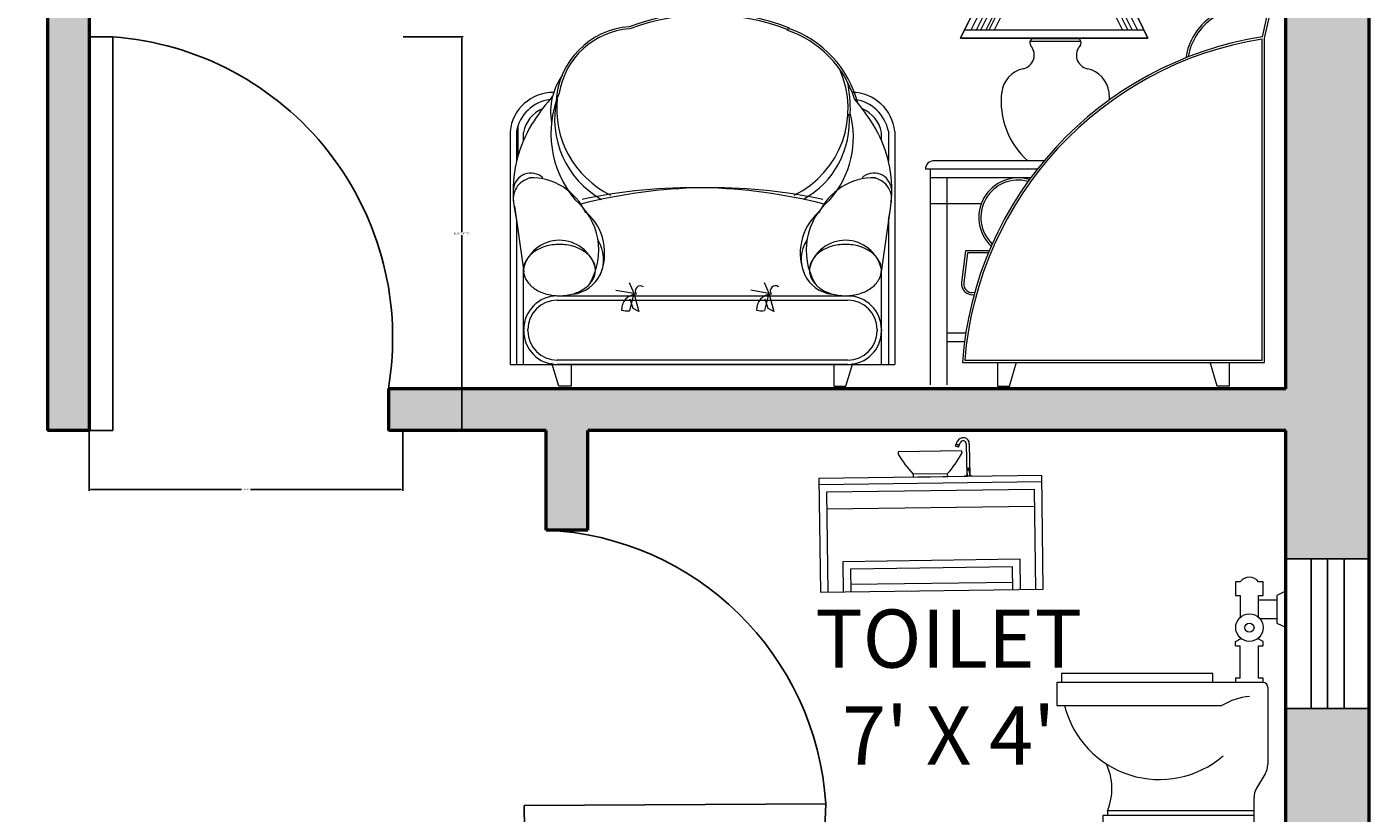
# Model space of a CAD drawing. Units: inches. Extents: x 1771 to 3025, y 319 to 889.
# Tile 30 of 35: x 2863 to 3025, y 619 to 714. Entities that reach past the tile are written whole.
import ezdxf

# ---------------------------------------------------------------- set-up
doc = ezdxf.new("R2010")
doc.units = ezdxf.units.IN
doc.header["$MEASUREMENT"] = 0
doc.set_wipeout_variables(frame=1)
for name, color, linetype, lineweight in [('A-ANNO-DIMS', 2, 'Continuous', 18), ('A-AREA-IDEN', 241, 'Continuous', 25), ('A-DOOR', 4, 'Continuous', 25), ('A-FLOR-FIXT', 8, 'Continuous', 18), ('A-FURN', 8, 'Continuous', 18), ('A-GLAZ', 40, 'Continuous', 25), ('A-WALL', 7, 'Continuous', 50), ('A-WALL-PATT', 254, 'Continuous', 13)]:
    doc.layers.add(name, color=color, linetype=linetype, lineweight=lineweight)
doc.styles.get("Standard").update_dxf_attribs({"font": 'arial.ttf'})
doc.dimstyles.get("Standard").update_dxf_attribs({"dimtxt": 0.18, "dimasz": 0.18, "dimexe": 0.18, "dimexo": 0.0625, "dimgap": 0.09, "dimtad": 0, "dimtih": 1, "dimtoh": 1, "dimdec": 4, "dimzin": 0, "dimdsep": 46, "dimtxsty": 'Standard', "dimcen": 0.09, "dimadec": 0, "dimazin": 0, "dimtfac": 1, "dimtdec": 4, "dimtofl": 0, "dimtmove": 0, "dimatfit": 3, "dimfxl": 1, "dimtolj": 1, "dimtzin": 0, "dimarcsym": 0})

# ---------------------------------------------------------------- blocks, each defined once
blk = doc.blocks.new('A$C425441F1')
for points in [[(1639.3, 0), (1667.3, 0), (1667.3, 55.3), (1748.6, 55.3), (1748.6, 807.4), (1761.1, 860.7), (1735.7, 880.7), (1703.4, 883.3), (1675.8, 879.6), (1656.2, 873.5), (1635.2, 863.3), (1619.6, 852.6), (1605.1, 839.5), (1596.7, 829.9), (1583.2, 810), (1573.2, 788.1), (1567.6, 767.7), (1566.5, 761.6), (1541.6, 750.9), (1510.7, 736.6), (1488.3, 725.3), (1464.5, 712.2), (1433.4, 693.6), (1409.1, 677.8), (1389.7, 664.2), (1388.2, 683.8), (1383.3, 700), (1376.2, 712), (1365.5, 723.2), (1352, 731.8), (1342.1, 735.4), (1331.7, 738.6), (1325, 742.7), (1317.7, 750.9), (1314.2, 758.8), (1312.9, 767.9), (1315.6, 780.8), (1321.1, 788.9), (1323.4, 793.7), (1323.6, 797.2), (1323.1, 800), (1320.5, 804.5), (1317.8, 806.7), (1317.8, 807.1), (1478.8, 807.1), (1345.8, 1080.7), (1177.3, 1080.7), (1044.3, 807.1), (1211.1, 807.1), (1211.1, 806.7), (1207.8, 803.9), (1205.8, 800.4), (1205.1, 796.3), (1207.6, 788.9), (1211.4, 783.4), (1213.5, 778.7), (1215.3, 769.8), (1215.1, 763.9), (1214.1, 759), (1208.8, 748.5), (1201.9, 741.7), (1195.3, 738), (1185.9, 735.4), (1176, 731.7), (1166.8, 726.4), (1159.9, 720.8), (1156.8, 717.7), (1149.3, 708.1), (1145.7, 701.6), (1143.6, 696.9), (1138.7, 669.7), (1138.7, 651.6), (1140.7, 631.8), (1142.6, 621.6), (1148.5, 600.5), (1162.8, 569), (1176.9, 547.8), (1188.6, 534.2), (1200, 523), (983, 523), (977.7, 522.3), (971.8, 519.6), (965.5, 512.8), (963.3, 506.8), (963, 503), (974.8, 503), (974.8, 3), (1013, 3), (1013, 103), (1053.6, 103), (1052.7, 96.1), (1051.6, 86.5), (1049.3, 63.6), (1048.6, 55.3), (1130.1, 55.3), (1130.1, 0), (1157.9, 0), (1174.1, 55.3), (1623.1, 55.6)], [(778.6, 0), (750.6, 0), (750.6, 50.4), (141.4, 50.4), (141.4, 0), (113.4, 0), (98.1, 50.4), (0, 50.4), (0, 590.4), (3.6, 609.1), (14.7, 633.7), (36.6, 658.7), (60.6, 673.3), (86.6, 680.5), (100.5, 681.5), (107.8, 698), (118.3, 717), (136.4, 751.3), (159.1, 779.5), (188.4, 803.6), (213.2, 817.4), (239.4, 827.1), (258.7, 831.4), (276, 833.4), (301.1, 842.1), (332.2, 850.9), (368.4, 858.6), (403.3, 863.5), (432.7, 865.8), (472.6, 866.2), (499.3, 864.8), (525, 862.1), (551.9, 857.9), (572.9, 853.6), (591.1, 849.1), (612.6, 842.8), (648, 830.4), (661.5, 823.7), (679.5, 815.2), (707.5, 798.2), (726.7, 783.3), (755.4, 754.4), (773.7, 729.8), (788.1, 704.9), (796.6, 686.1), (798.5, 681.2), (818, 677.9), (833.5, 672.3), (851.7, 661.6), (864.4, 650.3), (878.3, 632.1), (887.5, 611.7), (891.4, 595.2), (892, 590.4), (892, 50.4), (793.9, 50.4)]]:
    blk.add_wipeout(points)
for p, q in [((1044.3, 807.1), (1177.3, 1080.7)), ((1177.3, 1080.7), (1044.3, 807.1)), ((1188.8, 1068), (1069.3, 827.4)), ((1201.1, 1068), (1081.6, 827.4)), ((1211.2, 1068), (1091.7, 827.4)), ((1223.5, 1068), (1104, 827.4)), ((1230.5, 1068), (1110.9, 827.4)), ((1242.8, 1068), (1123.2, 827.4)), ((1171, 1067.8), (1351.9, 1067.8)), ((1177.3, 1080.7), (1345.8, 1080.7)), ((1345.8, 1080.7), (1177.3, 1080.7)), ((1299.6, 1068), (1419.2, 827.4)), ((1311.9, 1068), (1431.5, 827.4)), ((1322, 1068), (1441.5, 827.4)), ((1334.3, 1068), (1453.8, 827.4)), ((1345.8, 1080.7), (1478.8, 807.1)), ((1478.8, 807.1), (1345.8, 1080.7)), ((1733.6, 876.1), (1755.5, 858.7)), ((1735.7, 880.7), (1761.1, 860.7)), ((1744.1, 810.1), (1755.5, 858.7)), ((1748.6, 807.4), (1761.1, 860.7)), ((1053.8, 826.7), (1469.3, 826.7)), ((1478.8, 807.1), (1044.3, 807.1)), ((1044.3, 807.1), (1478.8, 807.1)), ((1205.6, 800), (1323.1, 800)), ((1211, 806.7), (1317.8, 806.7)), ((1743.6, 60.3), (1743.6, 805)), ((1748.6, 55.3), (1748.6, 807.4)), ((18.2, 603.6), (18.2, 536.8)), ((0, 590.4), (0, 50.4)), ((15, 591.1), (15, 521.6)), ((31, 569.9), (31, 588.4)), ((861, 569.9), (861, 588.4)), ((877, 591.1), (877, 521.6)), ((892, 590.4), (892, 50.4)), ((1222, 503), (963, 503)), ((974.8, 3), (974.8, 503)), ((1238.2, 523), (983, 523)), ((1206.8, 483), (974.8, 483)), ((1013, 3), (1013, 483)), ((10, 417.4), (32, 265.4)), ((882, 417.4), (860, 265.4)), ((1092.2, 423), (974.8, 423)), ((15, 385.1), (15, 50.4)), ((877, 385.1), (877, 50.4)), ((1055.6, 314.3), (1046.6, 240.3)), ((1111.1, 314.3), (1055.6, 314.3)), ((1060.1, 309.3), (1051.6, 239.7)), ((1109, 309.3), (1060.1, 309.3)), ((31, 50.4), (31, 272.3)), ((861, 50.4), (861, 272.3)), ((245.5, 223.1), (286.9, 216)), ((276.3, 240.8), (286.9, 216)), ((558.4, 223.2), (599.9, 216.1)), ((589.2, 240.9), (599.9, 216.1)), ((108.8, 209.4), (790.1, 209.4)), ((109.6, 209.4), (783, 209.4)), ((109.6, 199.4), (783, 199.4)), ((286.9, 216), (276.9, 175.2)), ((285.7, 179.9), (278.3, 201.7)), ((286.9, 216), (298.3, 173.5)), ((599.9, 216.1), (589.8, 175.3)), ((598.7, 180), (591.2, 201.8)), ((599.9, 216.1), (611.2, 173.6)), ((298.3, 173.5), (285.7, 179.9)), ((611.2, 173.6), (598.7, 180)), ((31.6, 128.4), (31.6, 131.4)), ((41.6, 128.4), (41.6, 131.4)), ((851, 131.4), (851, 128.4)), ((861, 131.4), (861, 128.4)), ((1056.5, 123), (1013, 123)), ((1053.6, 103), (1013, 103)), ((0, 50.4), (892, 50.4)), ((113.4, 0), (97.2, 53.4)), ((783, 60.4), (109.6, 60.4)), ((783, 50.4), (109.6, 50.4)), ((141.4, 50.4), (141.4, 0)), ((750.6, 50.4), (750.6, 0)), ((778.6, 0), (794.8, 53.4)), ((1048.6, 55.3), (1748.6, 55.3)), ((1054, 60.3), (1743.6, 60.3)), ((1129.9, 52.6), (1129.9, 0)), ((1157.9, 0), (1174.2, 55.6)), ((1639.3, 0), (1623.1, 55.6)), ((1667.3, 52.6), (1667.3, 0)), ((141.4, 0), (113.4, 0)), ((750.6, 0), (778.6, 0)), ((1129.9, 0), (1157.9, 0)), ((1667.3, 0), (1639.3, 0))]:
    blk.add_line(p, q)
for centre, radius, start, end in [((1708.4, 739.8), 143.6, 79.0486, 171.2543), ((1708.4, 739.8), 138.6, 79.5487, 170.0411), ((458.1, 348.7), 517.8, 68.4843, 110.5916), ((458.1, 348.7), 512.8, 68.4843, 110.5916), ((289.3, 651.4), 182.6, 93.9855, 176.965), ((289.3, 651.4), 177.6, 93.9855, 170.8791), ((563, 591.9), 246.9, 17.5917, 71.2419), ((563, 591.9), 251.9, 14.3659, 71.2419), ((1873.1, -6.5), 826.8, 98.9741, 175.711), ((1873.1, -6.5), 821.8, 99.0642, 175.3352), ((1183, 767.9), 32.3, 282.2329, 40.4775), ((1217.2, 796.3), 12.1, 120.8914, 217.6223), ((1345.2, 767.9), 32.3, 135.1029, 257.7671), ((1311.5, 796.3), 12.1, 322.3777, 59.1086), ((242.1, 635.9), 148, 144.2704, 189.5276), ((560.7, 643.7), 223.1, 296.1387, 23.9967), ((1203.5, 673.6), 64.2, 102.2329, 173.5671), ((1324.7, 673.6), 64.2, 6.4329, 77.7671), ((512.5, 645.7), 276.4, 357.4515, 12.4082), ((100.5, 580.5), 100.9, 89.5113, 174.4069), ((104.5, 574.5), 91, 97.7735, 169.4907), ((508.9, 316.7), 542.9, 139.0716, 146.5815), ((333.5, 586), 238.7, 156.9166, 219.7497), ((316.8, 619.2), 213.4, 167.2983, 240.5749), ((331.3, 643.7), 223.1, 173.6107, 243.8613), ((791.5, 580.5), 100.9, 5.5931, 89.1441), ((383.1, 316.7), 542.9, 33.4185, 40.1113), ((787.5, 574.5), 91, 10.5093, 82.2265), ((1322.1, 660.2), 183.7, 173.5671, 228.321), ((1206.1, 660.2), 183.7, 1.2452, 6.4329), ((104.5, 574.5), 74.8, 113.0142, 169.2704), ((579.4, 614.6), 207.2, 299.0365, 4.5654), ((578.1, 577), 217.9, 318.7723, 15.0106), ((787.5, 574.5), 74.8, 10.7296, 66.9858), ((301.8, 453.4), 294.8, 146.5815, 180), ((590.2, 453.4), 294.8, 0, 33.4185), ((983, 503), 20, 90, 180), ((56.7, 434.2), 49.4, 95.5103, 189.1585), ((48.3, 453.8), 40.5, 46.9039, 174.9451), ((49, 344.1), 139.3, 24.2628, 91.6479), ((843, 344.1), 139.3, 88.3521, 155.7372), ((843.7, 453.8), 40.5, 5.0549, 133.0961), ((835.3, 434.2), 49.4, 350.8415, 84.4897), ((1177.9, 391.7), 91.3, 73.3794, 227.0029), ((1177.9, 391.7), 86.3, 74.5383, 225.8439), ((301.8, 453.4), 294.8, 180, 193.379), ((468.1, -775.2), 1235.6, 77.9993, 104.2473), ((423.9, -775.2), 1235.6, 75.7527, 102.0007), ((590.2, 453.4), 294.8, 346.621, 0), ((52.4, 315.2), 153.2, 329.9033, 50.4478), ((839.6, 315.2), 153.2, 129.5522, 210.0967), ((92.5, 308.8), 126.8, 335.5815, 48.2351), ((799.5, 308.8), 126.8, 131.7649, 204.4185), ((114.7, 252.6), 85.8, 14.0074, 167.3648), ((93.5, 258.1), 65.5, 125.4727, 149.8309), ((106.2, 240.2), 87.4, 106.4444, 125.4727), ((114.5, 212.1), 116.8, 90, 106.4444), ((114.5, 212.1), 116.8, 73.5556, 90), ((135.5, 294.2), 81.5, 277.3995, 32.8179), ((122.8, 240.2), 87.4, 54.5273, 73.5556), ((135.5, 258.1), 65.5, 30.1691, 54.5273), ((756.5, 294.2), 81.5, 147.1821, 262.6005), ((777.3, 252.6), 85.8, 12.6352, 165.9926), ((756.5, 258.1), 65.5, 125.4727, 149.8309), ((769.2, 240.2), 87.4, 106.4444, 125.4727), ((777.5, 212.1), 116.8, 90, 106.4444), ((777.5, 212.1), 116.8, 73.5556, 90), ((785.8, 240.2), 87.4, 54.5273, 73.5556), ((798.5, 258.1), 65.5, 30.1691, 54.5273), ((74.1, 269.4), 43.1, 149.8309, 180), ((154.9, 269.4), 43.1, 0, 30.1691), ((737.1, 269.4), 43.1, 149.8309, 180), ((817.9, 269.4), 43.1, 0, 30.1691), ((74.1, 269.4), 43.1, 180, 210.1691), ((154.9, 269.4), 43.1, 329.8309, 0), ((737.1, 269.4), 43.1, 180, 210.1691), ((817.9, 269.4), 43.1, 329.8309, 0), ((93.5, 280.6), 65.5, 210.1691, 234.5273), ((106.2, 298.5), 87.4, 234.5273, 253.5556), ((122.8, 298.5), 87.4, 286.4444, 305.4727), ((135.5, 280.6), 65.5, 305.4727, 329.8309), ((302.4, 220.7), 12.2, 53.3958, 216.551), ((615.4, 220.8), 12.2, 53.3958, 216.551), ((756.5, 280.6), 65.5, 210.1691, 234.5273), ((769.2, 298.5), 87.4, 234.5273, 253.5556), ((785.8, 298.5), 87.4, 286.4444, 305.4727), ((798.5, 280.6), 65.5, 305.4727, 329.8309), ((1071.6, 237.3), 25.1, 173.0657, 279.7438), ((1071.6, 237.3), 20.1, 173.0657, 286.6808), ((109.6, 131.4), 78, 90, 180), ((109.6, 131.4), 68, 90, 180), ((114.5, 326.6), 116.8, 253.5556, 270), ((114.5, 326.6), 116.8, 270, 286.4444), ((294.4, 177.6), 35.9, 92.8846, 181.9), ((607.4, 177.7), 35.9, 92.8846, 181.9), ((777.5, 326.6), 116.8, 253.5556, 270), ((777.5, 326.6), 116.8, 270, 286.4444), ((783, 131.4), 78, 0, 90), ((783, 131.4), 68, 0, 90), ((271.5, 234.5), 59.6, 257.4358, 275.1883), ((584.4, 234.6), 59.6, 257.4358, 275.1883), ((109.6, 128.4), 78, 180, 270), ((109.6, 128.4), 68, 180, 270), ((783, 128.4), 68, 270, 0), ((783, 128.4), 78, 270, 0)]:
    blk.add_arc(centre, radius, start, end)
blk = doc.blocks.new('A$C062C426B')
for p, q in [((0.4867, 0.6739, -0.3429), (0.4867, 0.6365, -0.3429)), ((0.4992, 0.6739, -0.3429), (0.4867, 0.6739, -0.3429)), ((0.5616, 0.6739, -0.3429), (0.5491, 0.6739, -0.3429)), ((0.5616, 0.6365, -0.3429), (0.5616, 0.6739, -0.3429)), ((0.4867, 0.6365, -0.3429), (0.4992, 0.6365, -0.3429)), ((0.4992, 0.6365, -0.3429), (0.4992, 0.577, -0.3429)), ((0.5491, 0.6365, -0.3429), (0.5616, 0.6365, -0.3429)), ((0.5491, 0.577, -0.3429), (0.5491, 0.6365, -0.3429)), ((0.599, 0.624, -0.3429), (0.5491, 0.624, -0.3429)), ((0.624, 0.649, -0.3429), (0.599, 0.6365, -0.3429)), ((0.599, 0.6365, -0.3429), (0.599, 0.5616, -0.3429)), ((0.624, 0.5491, -0.3429), (0.624, 0.649, -0.3429)), ((0.5521, 0.5741, -0.3429), (0.599, 0.5741, -0.3429)), ((0.599, 0.5616, -0.3429), (0.624, 0.5491, -0.3429)), ((0.4867, 0.5117, -0.3429), (0.5017, 0.5192, -0.3429)), ((0.5616, 0.5117, -0.3429), (0.5466, 0.5192, -0.3429)), ((0.4867, 0.4992, -0.3429), (0.4867, 0.5117, -0.3429)), ((0.4867, 0.4992, -0.3429), (0.4992, 0.4992, -0.3429)), ((0.4992, 0.4118, -0.3429), (0.4992, 0.4992, -0.3429)), ((0.5491, 0.4118, -0.3429), (0.5491, 0.4992, -0.3429)), ((0.5491, 0.4992, -0.3429), (0.5616, 0.4992, -0.3429)), ((0.5616, 0.4992, -0.3429), (0.5616, 0.5117, -0.3429)), ((0.4243, 0.4243, -0.3429), (0.0125, 0.4243, -0.3429)), ((0.0125, 0.4243, -0.3429), (0.0125, 0.3994, -0.3429)), ((0.4243, 0.3994, -0.3429), (0.4243, 0.4243, -0.3429)), ((0.4992, 0.4118, -0.3429), (0.4867, 0.4118, -0.3429)), ((0.4867, 0.4118, -0.3429), (0.4867, 0.3994, -0.3429)), ((0.5616, 0.4118, -0.3429), (0.5491, 0.4118, -0.3429)), ((0.5616, 0.3994, -0.3429), (0.5616, 0.4118, -0.3429)), ((0.5616, 0.3994, -0.3429), (0, 0.3994, -0.3429)), ((0, 0.3994, -0.3429), (0, 0.337, -0.3429)), ((0.5741, 0.3869, -0.3429), (0.5741, 0.1761, -0.3429)), ((0, 0.337, -0.3429), (0.4493, 0.337, -0.3429)), ((0.567, 0.1504, -0.3429), (0.5438, 0.1117, -0.3429)), ((0.5366, 0.086, -0.3429), (0.5366, 0, -0.3429)), ((0.5366, 0.0374, -0.3429), (0.1248, 0.0374, -0.3429)), ((0.1248, 0.0374, -0.3429), (0.1248, 0, -0.3429)), ((0.5366, 0.0499, -0.3429), (0.1373, 0.0499, -0.3429)), ((0.1373, 0.0499, -0.3429), (0.1373, 0.0374, -0.3429))]:
    blk.add_line(p, q)
for radius in [0.0374, 0.0125]:
    blk.add_circle((0.5242, 0.5491, -0.3429), radius)
for centre, radius, start, end in [((0.5242, 0.6552, -0.3429), 0.0312, 36.8699, 143.1301), ((0.5616, 0.3869, -0.3429), 0.0125, 0, 90), ((0.2791, 0.4017, -0.3429), 0.2664, 194.0552, 310.7015), ((0.5429, 0.181, -0.3429), 0.1819, 95.9061, 120.9638), ((-0.0044, 0.1107, -0.3429), 0.1542, 336.7818, 25.8778), ((0.5242, 0.1761, -0.3429), 0.0499, 329.0362, 0), ((0.5866, 0.086, -0.3429), 0.0499, 149.0362, 180)]:
    blk.add_arc(centre, radius, start, end)
blk = doc.blocks.new('A$C127E6D2A')
for p, q in [((0.904, 0.9521), (0.9161, 0.9819)), ((0.9226, 0.9446), (0.9346, 0.9744)), ((0.525, 0.915), (0.525, 0.9063)), ((0.525, 0.915), (0.525, 0.9063)), ((0.94, 0.92), (0.53, 0.92)), ((0.9226, 0.9446), (0.904, 0.9521)), ((0.9275, 0.9563), (0.9088, 0.9639)), ((0.9282, 0.9582), (0.9095, 0.9657)), ((0.945, 0.915), (0.945, 0.9063)), ((0.975, 0.9647), (0.975, 0.756)), ((0.995, 0.964), (0.995, 0.756)), ((0.982, 0.8022), (0.982, 0.7905)), ((0.988, 0.8022), (0.988, 0.7905)), ((1.47, 0.75), (0, 0.75)), ((0, 0.75), (0, 0)), ((1.47, 0.71), (0, 0.71)), ((0.6225, 0.77), (0.6225, 0.75)), ((0.8475, 0.77), (0.6225, 0.77)), ((0.8475, 0.75), (0.6225, 0.75)), ((0.8475, 0.77), (0.8475, 0.75)), ((0.96, 0.756), (0.96, 0.75)), ((0.96, 0.756), (1.01, 0.756)), ((0.9925, 0.7905), (0.9775, 0.7905)), ((0.9775, 0.7905), (0.9775, 0.756)), ((0.9925, 0.7905), (0.9925, 0.756)), ((1.01, 0.756), (1.01, 0.75)), ((1.47, 0), (1.47, 0.75)), ((0.05, 0.66), (0.05, 0)), ((1.42, 0.66), (0.05, 0.66)), ((1.42, 0), (1.42, 0.66)), ((0.05, 0.55), (1.42, 0.55)), ((1.32, 0.2), (0.15, 0.2)), ((0.15, 0.2), (0.15, 0)), ((1.32, 0), (1.32, 0.2)), ((1.27, 0.15), (0.2, 0.15)), ((0.2, 0.15), (0.2, 0)), ((1.27, 0), (1.27, 0.15)), ((0.2, 0.05), (1.27, 0.05)), ((0, 0), (1.47, 0))]:
    blk.add_line(p, q)
blk.add_circle((0.985, 0.804), 0.0035)
for centre, radius, start, end in [((0.9541, 0.9665), 0.041, 356.58807, 157.98673), ((0.9541, 0.9665), 0.021, 355.23192, 157.98673), ((0.53, 0.915), 0.005, 90, 180), ((0.53, 0.9063), 0.005, 180, 209.45502), ((1.1676, 1.2664), 0.7372, 209.45502, 222.32259), ((0.3024, 1.2664), 0.7372, 317.67741, 330.54498), ((0.94, 0.915), 0.005, 0, 90), ((0.94, 0.9063), 0.005, 330.54498, 0)]:
    blk.add_arc(centre, radius, start, end)
blk = doc.blocks.new('DOOR-36B')
blk.add_lwpolyline([(0, 47.37), (2.84, 47.37), (2.84, 0), (0, 0)], close=True)
blk.add_arc((0.18, 11.12), 36.34, 350.3015, 85.8059)
blk = doc.blocks.new('DOOR-35')
blk.add_lwpolyline([(35.88, 36.19), (32.96, 36.3), (33.16, 0), (36, 0.05)], close=True)
blk.add_arc((35.23, 1.11), 35.26, 93.6879, 177.4925)
blk = doc.blocks.new('WIN-18')
for p, q in [((0, 0), (0, 10)), ((18, 0), (18, 10)), ((0, 7), (18, 7)), ((0, 5), (18, 5)), ((0, 3), (18, 3))]:
    blk.add_line(p, q)
blk = doc.blocks.new('*D28')
at = {"layer": 'A-ANNO-DIMS', "color": 0, "lineweight": -2, "transparency": 16777216}
for p, q in [((2908.47, 712.85), (2915.7, 712.85)), ((2915.52, 712.67), (2915.52, 689.35)), ((2915.52, 665.66), (2915.52, 688.98)), ((2908.47, 665.48), (2915.7, 665.48))]:
    blk.add_line(p, q, dxfattribs=at)
at = {"layer": 'A-ANNO-DIMS', "color": 0, "transparency": 16777216}
for points in [[(2915.49, 712.67), (2915.55, 712.67), (2915.52, 712.85)], [(2915.49, 665.66), (2915.55, 665.66), (2915.52, 665.48)]]:
    blk.add_solid(points, dxfattribs=at)
at = {"layer": 'Defpoints', "color": 0, "transparency": 16777216}
for p in [(2908.41, 712.85), (2915.52, 712.85), (2908.41, 665.48)]:
    blk.add_point(p, dxfattribs=at)
at = {"layer": 'A-ANNO-DIMS', "color": 0, "transparency": 16777216, "insert": (2915.52, 689.17), "char_height": 0.18, "attachment_point": 5}
blk.add_mtext('\\A1;DOOR D1 47 TYP.', dxfattribs=at)
blk = doc.blocks.new('*D29')
at = {"layer": 'A-ANNO-DIMS', "color": 0, "lineweight": -2, "transparency": 16777216}
for p, q in [((2870.68, 665.42), (2870.68, 658.2)), ((2908.41, 665.42), (2908.41, 658.2)), ((2870.86, 658.38), (2889.02, 658.38)), ((2908.23, 658.38), (2890.08, 658.38))]:
    blk.add_line(p, q, dxfattribs=at)
at = {"layer": 'A-ANNO-DIMS', "color": 0, "transparency": 16777216}
for points in [[(2870.86, 658.41), (2870.86, 658.35), (2870.68, 658.38)], [(2908.23, 658.41), (2908.23, 658.35), (2908.41, 658.38)]]:
    blk.add_solid(points, dxfattribs=at)
at = {"layer": 'Defpoints', "color": 0, "transparency": 16777216}
for p in [(2870.68, 665.48), (2908.41, 665.48), (2908.41, 658.38)]:
    blk.add_point(p, dxfattribs=at)
at = {"layer": 'A-ANNO-DIMS', "color": 0, "transparency": 16777216, "insert": (2889.55, 658.38), "char_height": 0.18, "attachment_point": 5}
blk.add_mtext('\\A1;38 TYP.', dxfattribs=at)

msp = doc.modelspace()

# ---------------------------------------------------------------- hatches: boundary and pattern name
at = {"layer": 'A-WALL-PATT'}
h = msp.add_hatch(color=256, dxfattribs=at)
h.dxf.hatch_style = 1
h.paths.add_polyline_path([(2870.68, 879.48), (2892.73, 879.48), (2892.73, 889.48), (2842.68, 889.48), (2842.68, 879.48), (2865.68, 879.48), (2865.68, 831.48), (2870.68, 831.48)])
h.paths.add_polyline_path([(2983.64, 889.48), (2940.73, 889.48), (2940.73, 879.48), (2961.68, 879.48), (2961.68, 795.48), (2865.68, 795.48), (2865.68, 759.48), (2865.68, 665.48), (2870.68, 665.48), (2870.68, 712.85), (2870.68, 790.48), (2978.68, 790.48), (2978.68, 795.48), (2966.68, 795.48), (2966.68, 879.48), (2983.64, 879.48)])
h.paths.add_polyline_path([(3024.68, 889.48), (3001.64, 889.48), (3001.64, 879.48), (3014.68, 879.48), (3014.68, 790.48), (3014.68, 769.46), (3024.68, 769.46)])
h.paths.add_polyline_path([(3024.68, 721.46), (3014.68, 721.46), (3014.68, 670.48), (2906.68, 670.48), (2906.68, 665.48), (2925.68, 665.48), (2925.68, 653.48), (2930.68, 653.48), (2930.68, 665.48), (3014.68, 665.48), (3014.68, 650.02), (3024.68, 650.02)])
h.paths.add_polyline_path([(3024.68, 632.02), (3014.68, 632.02), (3014.68, 617.48), (2925.68, 617.48), (2906.68, 617.48), (2906.68, 612.48), (3014.68, 612.48), (3014.68, 581.96), (3024.68, 581.96)])
h.paths.add_polyline_path([(3024.68, 533.96), (3014.68, 533.96), (3014.68, 480.48), (2870.68, 480.48), (2870.68, 617.48), (2860.68, 617.48), (2860.68, 544.48), (2769.68, 544.48), (2769.68, 534.48), (2860.68, 534.48), (2860.68, 470.48), (3014.68, 470.48), (3014.68, 453.61), (3024.68, 453.61)])
h.paths.add_polyline_path([(3024.68, 405.61), (3014.68, 405.61), (3014.68, 394.48), (2860.68, 394.48), (2860.68, 384.48), (3024.68, 384.48)])
h.paths.add_polyline_path([(2733.68, 643.43), (2723.68, 643.43), (2723.68, 534.48), (2733.68, 534.48)])
h.paths.add_polyline_path([(2733.68, 754.48), (2829.68, 754.48), (2829.68, 759.48), (2733.68, 759.48), (2733.68, 843.44, -0.008336), (2732.38, 843.48), (2723.68, 843.48), (2723.68, 691.43), (2733.68, 691.43)])
h.paths.add_polyline_path([(2794.68, 889.48), (2723.68, 889.48), (2723.68, 879.48), (2794.68, 879.48)])

# ---------------------------------------------------------------- linework, layer by layer
at = {"layer": 'A-WALL'}
for p, q in [((3024.68, 384.48), (3024.68, 889.28)), ((2870.68, 790.48), (2870.68, 670.48)), ((3014.68, 670.48), (3014.68, 790.48)), ((2865.68, 759.48), (2865.68, 665.48)), ((2870.68, 670.48), (2870.68, 665.48)), ((3014.68, 670.48), (2906.68, 670.48)), ((2906.68, 670.48), (2906.68, 665.48)), ((2870.68, 665.48), (2865.68, 665.48)), ((2925.68, 665.48), (2906.68, 665.48)), ((2925.68, 653.48), (2925.68, 665.48)), ((2930.68, 653.48), (2930.68, 665.48)), ((3014.68, 665.48), (2930.68, 665.48)), ((3014.68, 617.48), (3014.68, 665.48)), ((2930.68, 653.48), (2925.68, 653.48))]:
    msp.add_line(p, q, dxfattribs=at)

# ---------------------------------------------------------------- block references
at = {"layer": 'A-DOOR'}
msp.add_blockref('DOOR-36B', (2870.68, 665.48), dxfattribs=at)
at = {"layer": 'A-DOOR', "rotation": 269.9999999999965}
msp.add_blockref('DOOR-35', (2923.02, 653.48), dxfattribs=at)
at = {"layer": 'A-FLOR-FIXT', "xscale": 18.24536006826809, "yscale": 18.24536006826809, "zscale": 18.24536006826809, "rotation": 0.7699301504024306}
msp.add_blockref('A$C127E6D2A', (2958.66, 645.99, 15.15), dxfattribs=at)
at = {"layer": 'A-FLOR-FIXT', "xscale": 44.17762020618112, "yscale": 44.17762020618112, "zscale": 44.17762020618112}
msp.add_blockref('A$C062C426B', (2987.12, 617.48, 15.15), dxfattribs=at)
at = {"layer": 'A-GLAZ', "rotation": 270.0000000000004}
msp.add_blockref('WIN-18', (3014.69, 650.02), dxfattribs=at)

# ---------------------------------------------------------------- texts
at = {"layer": 'A-AREA-IDEN', "insert": (2931.36, 643.92), "char_height": 7, "attachment_point": 1}
msp.add_mtext_dynamic_manual_height_columns("\\pxqc;TOILET \\P7' X 4'", width=85.4611, gutter_width=1, heights=[0], dxfattribs=at)

# ---------------------------------------------------------------- dimensions: what is measured, and where the dimension line sits
at = {"layer": 'A-ANNO-DIMS'}
dim = msp.add_linear_dim(base=(2915.52, 712.85), p1=(2908.41, 665.48), p2=(2908.41, 712.85), angle=90, text='DOOR D1 <> TYP.', dimstyle='Standard', override={"dimdec": 0, "dimrnd": 0, "dimzin": 0, "dimlunit": 2}, dxfattribs=at)
dim.commit()
dim.dimension.update_dxf_attribs({"geometry": '*D28', "text_midpoint": (2915.52, 689.17)})
dim = msp.add_linear_dim(base=(2908.41, 658.38), p1=(2870.68, 665.48), p2=(2908.41, 665.48), text='<> TYP.', dimstyle='Standard', override={"dimdec": 0, "dimrnd": 0, "dimzin": 0, "dimlunit": 2}, dxfattribs=at)
dim.commit()
dim.dimension.update_dxf_attribs({"geometry": '*D29', "text_midpoint": (2889.55, 658.38)})

# ---------------------------------------------------------------- next in the draw order: block references
at = {"layer": 'A-FURN', "xscale": 0.0519011286993662, "yscale": 0.0519011286993662, "zscale": 0.0519011286993662}
msp.add_blockref('A$C425441F1', (2921.32, 670.79), dxfattribs=at)

doc.saveas('drawing.dxf')
